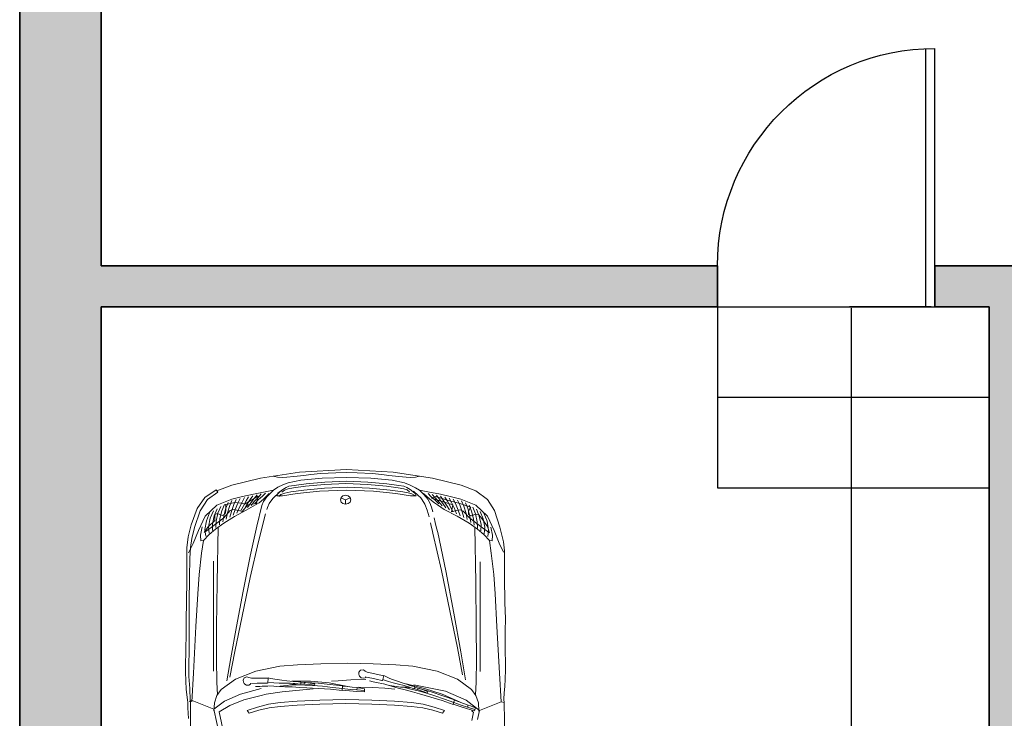
# Model space of a CAD drawing. Units: inches. Extents: x -5 to 482, y -460 to 66.
# Tile 9 of 31: x 33 to 142, y -329 to -252. Entities that reach past the tile are written whole.
import ezdxf

# ---------------------------------------------------------------- set-up
doc = ezdxf.new("R2010")
doc.units = ezdxf.units.IN
doc.header["$MEASUREMENT"] = 0
for name, color, linetype, lineweight in [('A-ANNO-DIMS', 2, 'Continuous', 18), ('A-DOOR', 3, 'Continuous', 25), ('A-EQPM-VEHI', 8, 'Continuous', 13), ('A-FLOR-STRS', 7, 'Continuous', 25), ('A-WALL', 7, 'Continuous', 35), ('A-WALL-PATT', 152, 'Continuous', 13)]:
    doc.layers.add(name, color=color, linetype=linetype, lineweight=lineweight)
doc.styles.get("Standard").update_dxf_attribs({"font": 'arial.ttf'})
doc.dimstyles.get("Standard").update_dxf_attribs({"dimtxt": 0.18, "dimasz": 0.18, "dimexe": 0.18, "dimexo": 0.0625, "dimgap": 0.09, "dimtad": 0, "dimtih": 1, "dimtoh": 1, "dimdec": 0, "dimzin": 0, "dimdsep": 46, "dimlunit": 3, "dimtxsty": 'Standard', "dimcen": 0.09, "dimadec": 0, "dimazin": 0, "dimtfac": 1, "dimtdec": 0, "dimtofl": 0, "dimtmove": 0, "dimatfit": 3, "dimfxl": 1, "dimtolj": 1, "dimtzin": 0, "dimarcsym": 0})

# ---------------------------------------------------------------- blocks, each defined once
blk = doc.blocks.new('*D18')
at = {"layer": 'A-ANNO-DIMS', "color": 0, "lineweight": -2, "transparency": 16777216}
for p, q in [((144.44, -144.35), (144.56, -144.35)), ((144.38, -144.53), (144.38, -208.69)), ((144.38, -279.17), (144.38, -215)), ((144.44, -279.35), (144.56, -279.35))]:
    blk.add_line(p, q, dxfattribs=at)
at = {"layer": 'A-ANNO-DIMS', "color": 0, "transparency": 16777216}
for points in [[(144.35, -144.53), (144.41, -144.53), (144.38, -144.35)], [(144.35, -279.17), (144.41, -279.17), (144.38, -279.35)]]:
    blk.add_solid(points, dxfattribs=at)
at = {"layer": 'Defpoints', "color": 0, "transparency": 16777216}
for p in [(144.38, -144.35), (144.38, -144.35), (144.38, -279.35)]:
    blk.add_point(p, dxfattribs=at)
at = {"layer": 'A-ANNO-DIMS', "color": 0, "transparency": 16777216, "insert": (144.38, -211.85), "char_height": 6, "attachment_point": 5}
blk.add_mtext('\\A1;11\'-3"', dxfattribs=at)
blk = doc.blocks.new('*D21')
at = {"layer": 'A-ANNO-DIMS', "color": 0, "lineweight": -2, "transparency": 16777216}
for p, q in [((133.45, -283.85), (124.45, -283.85)), ((124.63, -284.03), (124.63, -345.73)), ((124.63, -413.74), (124.63, -352.04)), ((124.69, -413.92), (124.81, -413.92))]:
    blk.add_line(p, q, dxfattribs=at)
at = {"layer": 'A-ANNO-DIMS', "color": 0, "transparency": 16777216}
for points in [[(124.6, -284.03), (124.66, -284.03), (124.63, -283.85)], [(124.6, -413.74), (124.66, -413.74), (124.63, -413.92)]]:
    blk.add_solid(points, dxfattribs=at)
at = {"layer": 'Defpoints', "color": 0, "transparency": 16777216}
for p in [(124.63, -283.85), (133.51, -283.85), (124.63, -413.92)]:
    blk.add_point(p, dxfattribs=at)
at = {"layer": 'A-ANNO-DIMS', "color": 0, "transparency": 16777216, "insert": (124.63, -348.88), "char_height": 6, "attachment_point": 5}
blk.add_mtext('\\A1;10\'-10"', dxfattribs=at)
blk = doc.blocks.new('DOOR-SWING-24IN')
for p, q in [((24, 1), (0, 1)), ((24, 0), (0, 0))]:
    blk.add_line(p, q)
blk.add_arc((24, 0), 24, 90, 180)

msp = doc.modelspace()

# ---------------------------------------------------------------- hatches: boundary and pattern name
at = {"layer": 'A-WALL-PATT'}
h = msp.add_hatch(color=256, dxfattribs=at)
h.dxf.hatch_style = 1
h.paths.add_polyline_path([(149.38, -412.85), (144.38, -412.85), (144.38, -283.85), (144.38, -279.35), (133.88, -279.35), (133.88, -283.85), (139.88, -283.85), (139.88, -412.85), (133.51, -412.85), (133.51, -413.92), (102.65, -413.92), (102.65, -421.02), (133.51, -421.02), (133.51, -421.85), (149.38, -421.85)])
h.paths.add_polyline_path([(226.05, -412.85), (218.88, -412.85), (218.88, -350.85), (262.88, -350.85), (262.88, -386.85), (267.38, -386.85), (267.38, -283.85), (270.38, -283.85), (270.38, -279.35), (244.88, -279.35), (244.88, -283.85), (262.88, -283.85), (262.88, -346.35), (218.88, -346.35), (218.88, -283.85), (220.88, -283.85), (220.88, -279.35), (214.38, -279.35), (214.38, -283.85), (214.38, -412.85), (209.38, -412.85), (209.38, -421.85), (226.05, -421.85)])
h.paths.add_polyline_path([(315.81, -412.85), (250.05, -412.85), (250.05, -421.85), (315.81, -421.85)])
h.paths.add_polyline_path([(430.38, -378.35), (421.38, -378.35), (421.38, -412.85), (375.81, -412.85), (375.81, -421.85), (430.38, -421.85)])
h.paths.add_polyline_path([(78.69, -413.92), (47.68, -413.92), (47.68, -412.85), (41.88, -412.85), (41.88, -283.85), (109.88, -283.85), (109.88, -279.35), (41.88, -279.35), (41.88, -241.85), (32.88, -241.85), (32.88, -421.85), (47.68, -421.85), (47.68, -421.02), (78.69, -421.02)])
h.paths.add_polyline_path([(41.88, -144.35), (154.38, -144.35), (154.38, -137.85), (149.88, -137.85), (149.88, -139.85), (41.88, -139.85), (41.88, -97.85), (32.88, -97.85), (32.88, -181.85), (41.88, -181.85)])
h.paths.add_polyline_path([(430.38, -241.85), (421.38, -241.85), (421.38, -279.35), (309.38, -279.35), (309.38, -170.35), (304.88, -170.35), (304.88, -279.35), (294.38, -279.35), (294.38, -283.85), (421.38, -283.85), (421.38, -318.35), (430.38, -318.35)])
h.paths.add_polyline_path([(430.38, -119.85), (421.38, -119.85), (421.38, -139.85), (419.38, -139.85), (419.38, -144.35), (421.38, -144.35), (421.38, -181.85), (430.38, -181.85)])
h.paths.add_polyline_path([(395.38, -139.85), (377.38, -139.85), (377.38, -75.85), (421.38, -75.85), (421.38, -95.85), (430.38, -95.85), (430.38, -45.6), (421.38, -45.6), (421.38, -71.35), (377.38, -71.35), (377.38, -22.85), (372.88, -22.85), (372.88, -139.85), (242.88, -139.85), (242.88, -137.85), (238.38, -137.85), (238.38, -144.35), (304.88, -144.35), (304.88, -146.35), (309.38, -146.35), (309.38, -144.35), (395.38, -144.35)])
h.paths.add_polyline_path([(65.88, 13.15), (32.88, 13.15), (32.88, -37.85), (41.88, -37.85), (41.88, 4.15), (65.88, 4.15)])
h.paths.add_polyline_path([(166.38, 13.15), (125.88, 13.15), (125.88, 4.15), (149.88, 4.15), (149.88, -113.85), (154.38, -113.85), (154.38, 4.15), (166.38, 4.15)])
h.paths.add_polyline_path([(277.88, 13.15), (226.38, 13.15), (226.38, 4.15), (238.38, 4.15), (238.38, -113.85), (242.88, -113.85), (242.88, 4.15), (277.88, 4.15)])
h.paths.add_polyline_path([(430.38, 13.15), (337.88, 13.15), (337.88, 4.15), (372.88, 4.15), (372.88, 1.15), (377.38, 1.15), (377.38, 4.15), (421.38, 4.15), (421.38, -21.6), (430.38, -21.6)])

# ---------------------------------------------------------------- linework, layer by layer
at = {"layer": 'A-DOOR'}
msp.add_line((132.88, -283.85), (132.88, -279.35), dxfattribs=at)
at = {"layer": 'A-EQPM-VEHI'}
for p, q in [((68.93, -301.81), (63.77, -302.12)), ((68.93, -301.81), (74.1, -302.12)), ((59.45, -302.78), (56.29, -303.55)), ((63.77, -302.12), (59.45, -302.78)), ((60.86, -302.56), (61.32, -302.65)), ((61.32, -302.65), (61.86, -302.68)), ((61.86, -302.68), (62.35, -302.66)), ((62.35, -302.66), (63.14, -302.58)), ((62.52, -303.27), (63.89, -303)), ((63.14, -302.58), (64.25, -302.46)), ((63.89, -303), (66.26, -302.78)), ((64.25, -302.46), (65.02, -302.36)), ((65.02, -302.36), (66.08, -302.27)), ((66.08, -302.27), (67.76, -302.19)), ((66.26, -302.78), (68.93, -302.69)), ((66.56, -303.2), (68.93, -303.1)), ((67.76, -302.19), (68.93, -302.15)), ((70.11, -302.19), (68.93, -302.15)), ((68.93, -302.69), (71.61, -302.78)), ((68.93, -303.1), (71.31, -303.2)), ((71.79, -302.27), (70.11, -302.19)), ((71.61, -302.78), (73.98, -303)), ((72.85, -302.36), (71.79, -302.27)), ((73.62, -302.46), (72.85, -302.36)), ((74.73, -302.58), (73.62, -302.46)), ((73.98, -303), (75.35, -303.27)), ((74.1, -302.12), (78.42, -302.78)), ((75.52, -302.66), (74.73, -302.58)), ((76.01, -302.68), (75.52, -302.66)), ((76.55, -302.65), (76.01, -302.68)), ((77.01, -302.56), (76.55, -302.65)), ((78.42, -302.78), (81.58, -303.55)), ((53.32, -304.91), (54.57, -304.06)), ((54.57, -304.06), (54.74, -304.3)), ((56.29, -303.55), (54.64, -304.18)), ((60.89, -304.11), (60.14, -304.83)), ((60.16, -304.25), (60.89, -304.11)), ((60.89, -304.11), (61.36, -303.77)), ((61.36, -303.77), (61.9, -303.51)), ((61.37, -304.42), (61.91, -304.01)), ((61.82, -304.33), (62.1, -304.09)), ((61.9, -303.51), (62.52, -303.27)), ((61.91, -304.01), (62.27, -303.79)), ((62.1, -304.09), (62.49, -303.94)), ((62.27, -303.79), (62.59, -303.66)), ((62.49, -303.94), (63.11, -303.83)), ((62.59, -303.66), (63.16, -303.57)), ((62.81, -304.29), (64.24, -304.11)), ((63.11, -303.83), (64.42, -303.66)), ((63.16, -303.57), (64.48, -303.4)), ((65.96, -304.22), (63.51, -304.47)), ((64.24, -304.11), (66.53, -303.87)), ((64.42, -303.66), (66.51, -303.46)), ((64.48, -303.4), (66.56, -303.2)), ((68.9, -304.11), (65.96, -304.22)), ((66.51, -303.46), (68.88, -303.36)), ((66.53, -303.87), (69.01, -303.75)), ((68.88, -303.36), (71.26, -303.46)), ((71.91, -304.22), (68.9, -304.11)), ((69.01, -303.75), (71.49, -303.87)), ((71.26, -303.46), (73.34, -303.66)), ((71.31, -303.2), (73.39, -303.4)), ((71.49, -303.87), (73.75, -304.11)), ((74.37, -304.47), (71.91, -304.22)), ((73.34, -303.66), (74.66, -303.83)), ((73.39, -303.4), (74.71, -303.57)), ((73.75, -304.11), (75.17, -304.29)), ((74.66, -303.83), (75.26, -303.93)), ((74.71, -303.57), (75.28, -303.66)), ((75.26, -303.93), (75.62, -304.06)), ((75.28, -303.66), (75.6, -303.79)), ((75.35, -303.27), (75.98, -303.54)), ((75.6, -303.79), (75.96, -304.01)), ((75.62, -304.06), (75.89, -304.26)), ((75.96, -304.01), (76.5, -304.42)), ((75.98, -303.54), (76.54, -303.82)), ((76.35, -304.2), (76.82, -304.63)), ((76.54, -303.82), (76.98, -304.11)), ((76.98, -304.11), (77.44, -304.55)), ((76.98, -304.11), (77.9, -304.28)), ((81.58, -303.55), (83.23, -304.18)), ((83.23, -304.18), (84.49, -305.12)), ((52.46, -306.1), (53.32, -304.91)), ((53.59, -305.14), (52.79, -306.38)), ((54.74, -304.3), (53.59, -305.14)), ((54.65, -305.76), (56.3, -305.09)), ((56.28, -305.23), (56.05, -305.79)), ((56.3, -305.09), (57.48, -304.79)), ((56.75, -305.12), (56.5, -305.66)), ((57.21, -305.02), (56.95, -305.53)), ((57.68, -304.92), (57.41, -305.4)), ((57.48, -304.79), (58.67, -304.54)), ((57.86, -305.27), (57.52, -305.88)), ((57.68, -305.63), (59.19, -304.75)), ((58.14, -304.82), (57.86, -305.27)), ((58.31, -305.14), (57.95, -305.69)), ((58.6, -304.71), (58.31, -305.14)), ((58.77, -305.01), (58.37, -305.51)), ((58.8, -305.32), (58.43, -305.78)), ((58.67, -304.54), (60.16, -304.25)), ((59.07, -304.61), (58.77, -305.01)), ((59.22, -304.88), (58.8, -305.32)), ((59.23, -305.14), (58.82, -305.57)), ((59.19, -304.75), (59, -305.55)), ((59.53, -304.51), (59.22, -304.88)), ((59.67, -304.75), (59.23, -305.14)), ((59.31, -305.48), (59.79, -305.1)), ((60, -304.41), (59.67, -304.75)), ((60.14, -304.83), (59.77, -305.35)), ((59.79, -305.1), (60.42, -304.48)), ((60.82, -305), (60.4, -305.57)), ((61.6, -304.29), (60.82, -305)), ((61.24, -304.72), (61.37, -304.42)), ((61.87, -304.72), (61.24, -304.72)), ((61.46, -304.8), (61.69, -304.58)), ((61.69, -304.58), (62.14, -304.42)), ((63.51, -304.47), (61.87, -304.72)), ((62.14, -304.42), (62.81, -304.29)), ((68.27, -305.15), (68.34, -304.9)), ((68.34, -305.4), (68.27, -305.15)), ((68.84, -305.15), (68.32, -304.93)), ((68.34, -304.9), (68.55, -304.72)), ((68.55, -304.72), (68.84, -304.65)), ((68.84, -304.65), (69.12, -304.72)), ((69.35, -304.93), (68.84, -305.15)), ((68.84, -305.15), (68.84, -305.65)), ((69.12, -304.72), (69.33, -304.9)), ((69.33, -304.9), (69.41, -305.15)), ((69.41, -305.15), (69.33, -305.4)), ((76, -304.72), (74.37, -304.47)), ((75.17, -304.29), (75.74, -304.39)), ((75.74, -304.39), (76.15, -304.5)), ((76.62, -304.72), (76, -304.72)), ((76.15, -304.5), (76.49, -304.68)), ((76.5, -304.42), (76.62, -304.72)), ((76.82, -304.63), (77.14, -304.94)), ((77.14, -304.94), (77.31, -305.17)), ((77.31, -305.17), (77.57, -305.65)), ((77.44, -304.55), (77.75, -304.86)), ((78.13, -305.1), (77.45, -304.48)), ((77.75, -304.86), (77.92, -305.09)), ((77.9, -304.28), (79.3, -304.55)), ((77.92, -305.09), (78.14, -305.5)), ((77.94, -304.46), (78.26, -304.8)), ((78.65, -305.48), (78.13, -305.1)), ((78.26, -304.8), (78.71, -305.19)), ((78.75, -304.8), (78.34, -304.98)), ((78.34, -304.98), (80.67, -305.7)), ((78.4, -304.56), (78.72, -304.93)), ((78.71, -305.19), (79.12, -305.62)), ((78.72, -304.93), (79.14, -305.38)), ((80.47, -305.3), (78.75, -304.8)), ((78.87, -304.66), (79.17, -305.06)), ((79.17, -305.06), (79.56, -305.56)), ((79.3, -304.55), (80.39, -304.79)), ((79.33, -304.77), (79.62, -305.19)), ((79.62, -305.19), (79.99, -305.74)), ((79.8, -304.87), (80.08, -305.32)), ((80.08, -305.32), (80.42, -305.93)), ((80.26, -304.97), (80.53, -305.45)), ((80.39, -304.79), (81.57, -305.09)), ((80.78, -305.38), (80.47, -305.3)), ((80.73, -305.07), (80.98, -305.58)), ((81.19, -305.18), (81.44, -305.72)), ((81.57, -305.09), (83.22, -305.76)), ((81.65, -305.28), (81.89, -305.85)), ((84.49, -305.12), (85.26, -306.35)), ((51.81, -307.91), (52.46, -306.1)), ((52.79, -306.38), (52.16, -308.21)), ((53.36, -306.98), (54.65, -305.76)), ((54.25, -306.37), (53.9, -307.2)), ((54.66, -306.14), (54.33, -306.92)), ((55.06, -305.91), (54.76, -306.64)), ((55.19, -306.36), (54.98, -307.22)), ((55.47, -305.69), (55.19, -306.36)), ((55.62, -306.08), (55.39, -306.92)), ((56.1, -306.35), (55.4, -307.14)), ((55.54, -306.72), (55.61, -306.32)), ((55.6, -305.68), (56.67, -305.46)), ((55.61, -305.89), (55.6, -305.68)), ((55.61, -306.32), (55.61, -305.89)), ((55.88, -305.46), (55.62, -306.08)), ((56.05, -305.79), (55.81, -306.61)), ((56.4, -306.21), (56.1, -306.35)), ((56.5, -305.66), (56.24, -306.43)), ((57.05, -306.34), (56.4, -306.21)), ((56.66, -306.24), (56.45, -306.85)), ((56.6, -307.01), (57.87, -306.3)), ((56.95, -305.53), (56.66, -306.24)), ((56.67, -305.46), (57.41, -305.54)), ((57.09, -306.06), (56.85, -306.64)), ((57.42, -306.44), (57.05, -306.34)), ((57.41, -305.4), (57.09, -306.06)), ((57.52, -305.88), (57.24, -306.42)), ((57.41, -305.54), (57.68, -305.63)), ((58.04, -305.73), (57.42, -306.44)), ((57.95, -305.69), (57.64, -306.21)), ((57.87, -306.3), (58.9, -305.73)), ((58.37, -305.51), (58.03, -306)), ((59, -305.55), (58.04, -305.73)), ((58.9, -305.73), (59.31, -305.48)), ((59.6, -305.78), (59.03, -308.05)), ((59.77, -305.35), (59.6, -305.78)), ((60.21, -306.01), (60.14, -306.22)), ((60.4, -305.57), (60.21, -306.01)), ((68.55, -305.58), (68.34, -305.4)), ((68.84, -305.65), (68.55, -305.58)), ((69.12, -305.58), (68.84, -305.65)), ((69.33, -305.4), (69.12, -305.58)), ((77.57, -305.65), (77.84, -306.3)), ((77.84, -306.3), (78.05, -307.03)), ((78.14, -305.5), (78.32, -305.96)), ((78.32, -305.96), (78.48, -306.47)), ((78.97, -305.73), (78.65, -305.48)), ((79.73, -306.21), (78.97, -305.73)), ((79.14, -305.38), (79.51, -305.83)), ((79.56, -305.56), (79.9, -306.05)), ((81.14, -306.96), (79.73, -306.21)), ((79.99, -305.74), (80.3, -306.26)), ((80.42, -305.93), (80.69, -306.48)), ((80.67, -305.7), (80.52, -306.5)), ((80.52, -306.5), (80.88, -306.39)), ((80.53, -305.45), (80.85, -306.11)), ((81.57, -305.6), (80.78, -305.38)), ((80.85, -306.11), (81.09, -306.69)), ((80.88, -306.39), (81.54, -306.27)), ((80.98, -305.58), (81.27, -306.29)), ((81.27, -306.29), (81.48, -306.91)), ((81.44, -305.72), (81.7, -306.48)), ((81.54, -306.27), (81.83, -306.4)), ((82.67, -305.98), (81.57, -305.6)), ((81.83, -306.4), (82.54, -307.19)), ((81.89, -305.85), (82.13, -306.66)), ((82.06, -305.51), (82.32, -306.13)), ((82.32, -306.13), (82.54, -306.97)), ((82.41, -306.44), (82.57, -306.12)), ((82.47, -305.74), (82.75, -306.41)), ((82.57, -306.12), (82.67, -305.98)), ((82.75, -306.41), (82.96, -307.27)), ((82.87, -305.97), (83.18, -306.69)), ((83.22, -305.76), (84.51, -306.98)), ((83.28, -306.2), (83.6, -306.97)), ((85.26, -306.35), (85.86, -308.17)), ((52.61, -308.55), (53.36, -306.98)), ((53.48, -307.48), (53.32, -308.44)), ((53.84, -306.6), (53.48, -307.48)), ((53.63, -308.16), (54.42, -307.43)), ((53.9, -307.2), (53.73, -308.14)), ((55.4, -307.14), (53.99, -308.21)), ((54.33, -306.92), (54.15, -307.83)), ((54.4, -306.77), (54.72, -306.68)), ((54.42, -307.43), (54.4, -306.77)), ((54.76, -306.64), (54.56, -307.53)), ((54.72, -306.68), (55.22, -306.88)), ((54.98, -307.22), (54.91, -307.91)), ((55.22, -306.88), (55.54, -306.72)), ((55.39, -306.92), (55.29, -307.6)), ((55.39, -307.73), (56.6, -307.01)), ((55.81, -306.61), (55.67, -307.28)), ((56.24, -306.43), (56.06, -307.07)), ((59.99, -306.7), (59.22, -309.74)), ((78.63, -307.16), (78.74, -307.66)), ((82.48, -307.73), (81.14, -306.96)), ((81.7, -306.48), (81.88, -307.12)), ((82.13, -306.66), (82.27, -307.34)), ((82.4, -306.77), (82.41, -306.44)), ((82.71, -306.93), (82.4, -306.77)), ((82.54, -306.97), (82.65, -307.65)), ((82.54, -307.19), (83.95, -308.26)), ((83.22, -306.74), (82.71, -306.93)), ((82.96, -307.27), (83.02, -307.96)), ((83.18, -306.69), (83.37, -307.58)), ((83.54, -306.82), (83.22, -306.74)), ((83.89, -307.23), (83.54, -306.82)), ((83.6, -306.97), (83.79, -307.88)), ((83.69, -306.43), (84.03, -307.25)), ((84.5, -308.09), (83.89, -307.23)), ((84.03, -307.25), (84.21, -308.19)), ((84.09, -306.65), (84.46, -307.53)), ((84.51, -306.98), (85.24, -308.54)), ((51.48, -309.25), (51.81, -307.91)), ((52.16, -308.21), (51.87, -309.42)), ((52.01, -309.98), (52.61, -308.55)), ((53.01, -308.14), (52.82, -309.05)), ((53.22, -308.75), (53.63, -308.16)), ((53.99, -308.21), (53.22, -308.75)), ((53.32, -308.44), (53.41, -309.16)), ((53.73, -308.14), (53.78, -308.85)), ((53.78, -309), (54.47, -308.38)), ((54.15, -307.83), (54.16, -308.53)), ((54.47, -308.38), (55.39, -307.73)), ((54.56, -307.53), (54.54, -308.22)), ((54.78, -308.17), (54.66, -314.28)), ((59.03, -308.05), (58.31, -311.37)), ((78.21, -307.71), (78.29, -308.08)), ((78.29, -308.08), (78.38, -308.46)), ((78.38, -308.46), (78.47, -308.83)), ((78.74, -307.66), (78.89, -308.27)), ((78.89, -308.27), (79.01, -308.77)), ((83.4, -308.38), (82.48, -307.73)), ((83.09, -308.17), (83.2, -314.28)), ((83.37, -307.58), (83.4, -308.27)), ((84.09, -309), (83.4, -308.38)), ((83.79, -307.88), (83.78, -308.59)), ((83.95, -308.26), (84.72, -308.8)), ((84.21, -308.19), (84.15, -308.9)), ((84.46, -307.53), (84.62, -308.49)), ((84.72, -308.8), (84.5, -308.09)), ((84.62, -308.49), (84.53, -309.21)), ((84.87, -308.17), (85.05, -309.07)), ((85.24, -308.54), (85.8, -309.93)), ((85.86, -308.17), (86.27, -309.81)), ((51.33, -310.47), (51.48, -309.25)), ((51.87, -309.42), (51.74, -310.43)), ((52.82, -309.05), (52.85, -309.68)), ((52.85, -309.68), (53.16, -309.65)), ((53.16, -309.65), (52.95, -311.05)), ((53.16, -309.65), (53.78, -309)), ((78.47, -308.83), (79.41, -312.97)), ((79.01, -308.77), (79.89, -313.01)), ((84.71, -309.65), (84.09, -309)), ((84.71, -309.65), (84.92, -311.05)), ((85.01, -309.69), (84.71, -309.65)), ((85.05, -309.07), (85.01, -309.69)), ((51.31, -311.81), (51.33, -310.47)), ((51.5, -311), (52.01, -309.98)), ((51.74, -310.43), (51.66, -311.64)), ((59.22, -309.74), (58.31, -313.72)), ((85.8, -309.93), (86.28, -310.95)), ((86.27, -309.81), (86.39, -310.77)), ((51.31, -313.83), (51.31, -311.81)), ((51.66, -311.64), (51.61, -313.7)), ((52.95, -311.05), (52.68, -313.41)), ((58.31, -311.37), (57.54, -315.23)), ((84.92, -311.05), (85.19, -313.41)), ((86.39, -310.77), (86.37, -311.65)), ((86.37, -311.65), (86.38, -313.71)), ((54.25, -324.05), (54.25, -311.91)), ((83.71, -324.09), (83.71, -311.99)), ((51.27, -316.59), (51.31, -313.83)), ((51.61, -313.7), (51.58, -316.54)), ((52.68, -313.41), (52.52, -315.53)), ((58.31, -313.72), (57.41, -317.99)), ((79.41, -312.97), (80.36, -317.42)), ((79.89, -313.01), (80.78, -317.67)), ((85.19, -313.41), (85.35, -315.53)), ((86.38, -313.71), (86.43, -316.54)), ((54.66, -314.28), (54.6, -319.13)), ((83.2, -314.28), (83.26, -319.13)), ((52.52, -315.53), (52.33, -319.12)), ((57.54, -315.23), (56.8, -319.15)), ((85.35, -315.53), (85.54, -319.12)), ((51.24, -318.27), (51.27, -316.59)), ((51.58, -316.54), (51.57, -318.27)), ((86.43, -316.54), (86.47, -318.27)), ((51.24, -319.71), (51.24, -318.27)), ((51.57, -318.27), (51.57, -319.7)), ((57.41, -317.99), (56.61, -321.89)), ((80.36, -317.42), (81.18, -321.49)), ((80.78, -317.67), (81.55, -321.95)), ((86.47, -318.27), (86.46, -319.66)), ((52.33, -319.12), (52.04, -324.3)), ((54.6, -319.13), (54.59, -322.77)), ((56.8, -319.15), (56.17, -322.61)), ((83.26, -319.13), (83.27, -322.77)), ((85.54, -319.12), (85.83, -324.3)), ((51.22, -321.92), (51.24, -319.71)), ((51.57, -319.7), (51.57, -321.9)), ((86.46, -319.66), (86.45, -321.79)), ((81.18, -321.49), (81.75, -324.48)), ((51.19, -323.33), (51.22, -321.92)), ((51.57, -321.9), (51.55, -323.31)), ((56.17, -322.61), (55.74, -325.14)), ((56.61, -321.89), (56.05, -324.74)), ((81.55, -321.95), (82.07, -325.04)), ((86.45, -321.79), (86.47, -323.17)), ((51.18, -324.13), (51.19, -323.33)), ((51.55, -323.31), (51.55, -324.65)), ((54.59, -322.77), (54.63, -325.27)), ((61.59, -323.5), (58.93, -324.06)), ((63.52, -323.35), (61.59, -323.5)), ((66.11, -323.26), (63.52, -323.35)), ((69.03, -323.18), (66.11, -323.26)), ((71.9, -323.26), (69.03, -323.18)), ((74.39, -323.35), (71.9, -323.26)), ((76.28, -323.5), (74.39, -323.35)), ((78.94, -324.06), (76.28, -323.5)), ((83.27, -322.77), (83.24, -325.27)), ((86.47, -323.17), (86.48, -323.93)), ((51.2, -325.18), (51.18, -324.13)), ((51.55, -324.65), (51.65, -325.96)), ((52.04, -324.3), (51.87, -327.46)), ((58.93, -324.06), (56.68, -324.96)), ((57.52, -325.07), (57.64, -324.81)), ((57.64, -324.81), (57.96, -324.69)), ((57.96, -324.69), (58.18, -324.78)), ((58.18, -324.78), (58.44, -324.85)), ((58.44, -324.85), (60.3, -324.84)), ((60.31, -324.81), (60.27, -325.4)), ((60.55, -324.86), (60.31, -324.81)), ((60.8, -324.92), (60.55, -324.86)), ((70.29, -324.39), (70.3, -324.18)), ((70.33, -324.53), (70.29, -324.39)), ((70.3, -324.18), (70.47, -323.95)), ((70.39, -324.63), (70.33, -324.53)), ((70.55, -324.79), (70.39, -324.63)), ((70.47, -323.95), (70.81, -323.91)), ((70.82, -324.85), (70.55, -324.79)), ((70.81, -323.91), (71, -324.05)), ((71, -324.79), (70.82, -324.85)), ((71, -324.05), (71.24, -324.17)), ((71.03, -324.73), (71, -324.79)), ((71.06, -324.7), (71.03, -324.73)), ((71.75, -324.85), (71.11, -324.72)), ((71.24, -324.17), (73.06, -324.58)), ((72.22, -324.95), (71.75, -324.85)), ((73.07, -324.55), (72.9, -325.12)), ((73.36, -324.68), (73.07, -324.55)), ((73.71, -324.86), (73.36, -324.68)), ((74, -324.98), (73.71, -324.86)), ((81.19, -324.96), (78.94, -324.06)), ((85.83, -324.3), (86, -327.46)), ((86.48, -323.93), (86.46, -324.94)), ((51.26, -326.04), (51.2, -325.18)), ((51.65, -325.96), (51.7, -327.3)), ((54.63, -325.27), (54.71, -326.68)), ((56.68, -324.96), (55.12, -326.07)), ((59.53, -325.96), (57.23, -326.59)), ((57.56, -325.28), (57.52, -325.07)), ((57.64, -325.41), (57.56, -325.28)), ((57.71, -325.49), (57.64, -325.41)), ((57.9, -325.61), (57.71, -325.49)), ((58.18, -325.6), (57.9, -325.61)), ((58.34, -325.5), (58.18, -325.6)), ((58.36, -325.44), (58.34, -325.5)), ((58.38, -325.41), (58.36, -325.44)), ((59.08, -325.4), (58.44, -325.41)), ((58.9, -325.75), (59.14, -325.75)), ((59.57, -325.39), (59.08, -325.4)), ((59.14, -325.75), (59.39, -325.74)), ((59.39, -325.74), (59.63, -325.73)), ((60.21, -325.38), (59.57, -325.39)), ((59.63, -325.73), (59.84, -325.72)), ((59.84, -325.72), (60.06, -325.72)), ((60.06, -325.72), (60.27, -325.71)), ((60.35, -325.7), (62.15, -325.8)), ((60.94, -325.34), (60.36, -325.3)), ((61.04, -324.96), (60.8, -324.92)), ((61.5, -325.38), (60.94, -325.34)), ((61.79, -325.06), (61.04, -324.96)), ((61.21, -325.74), (62.38, -325.63)), ((62.08, -325.38), (61.5, -325.38)), ((62.36, -325.14), (61.79, -325.06)), ((62.72, -325.38), (62.08, -325.38)), ((62.15, -325.8), (62.96, -325.81)), ((63.06, -325.2), (62.36, -325.14)), ((62.71, -325.57), (62.38, -325.63)), ((63.52, -325.59), (62.69, -325.57)), ((63.04, -325.5), (62.71, -325.57)), ((63.24, -325.42), (62.72, -325.38)), ((64.97, -325.18), (62.9, -325.16)), ((62.96, -325.81), (63.77, -325.85)), ((63.37, -325.48), (63.04, -325.5)), ((63.34, -325.22), (63.06, -325.2)), ((63.89, -325.5), (63.24, -325.42)), ((63.63, -325.25), (63.34, -325.22)), ((64.36, -325.6), (63.52, -325.59)), ((63.91, -325.27), (63.63, -325.25)), ((63.77, -325.85), (64.57, -325.9)), ((63.88, -325.46), (64.4, -325.49)), ((63.91, -325.29), (63.89, -325.5)), ((64.41, -325.31), (63.9, -325.28)), ((64.3, -325.3), (64.28, -325.48)), ((65.19, -325.63), (64.36, -325.6)), ((64.4, -325.49), (64.91, -325.55)), ((64.93, -325.38), (64.41, -325.31)), ((64.45, -325.33), (65.8, -325.39)), ((64.57, -325.9), (65.87, -325.96)), ((64.91, -325.55), (65.42, -325.62)), ((65.44, -325.45), (64.93, -325.38)), ((67.04, -325.36), (64.97, -325.18)), ((66.29, -325.73), (65.19, -325.63)), ((65.44, -325.45), (65.41, -325.62)), ((65.8, -325.39), (67.15, -325.53)), ((65.87, -325.96), (67.18, -326.05)), ((67.39, -325.85), (66.29, -325.73)), ((69.08, -325.77), (67.04, -325.36)), ((67.15, -325.53), (68.5, -325.68)), ((68.03, -325.12), (67.28, -325.16)), ((68.49, -325.96), (67.39, -325.85)), ((69.43, -325.04), (68.03, -325.12)), ((68.5, -325.68), (68.48, -326.16)), ((69.37, -326.08), (68.48, -325.97)), ((68.5, -325.72), (69.04, -325.77)), ((69.04, -325.77), (69.57, -325.82)), ((71.06, -324.99), (69.43, -325.04)), ((69.57, -325.82), (70.11, -325.88)), ((70.11, -325.89), (70.09, -326.13)), ((70.11, -325.89), (70.39, -325.92)), ((71.82, -325.85), (70.3, -325.82)), ((70.39, -325.92), (70.66, -325.96)), ((70.66, -325.96), (70.94, -326)), ((71.49, -325.15), (71.89, -325.24)), ((73.16, -325.93), (71.82, -325.85)), ((71.89, -325.24), (72.44, -325.35)), ((72.85, -325.08), (72.22, -324.95)), ((72.44, -325.35), (72.83, -325.42)), ((72.92, -325.43), (74.65, -325.93)), ((73.57, -325.21), (73.01, -325.04)), ((74.29, -326.04), (73.16, -325.93)), ((74.1, -325.37), (73.57, -325.21)), ((73.74, -325.66), (74.91, -325.82)), ((74.58, -325.17), (74, -324.98)), ((74.67, -325.51), (74.1, -325.37)), ((75.08, -325.36), (74.58, -325.17)), ((74.65, -325.93), (75.43, -326.12)), ((75.3, -325.65), (74.67, -325.51)), ((75.24, -325.83), (74.91, -325.82)), ((75.67, -325.55), (75.08, -325.36)), ((76.03, -326.04), (75.22, -325.83)), ((75.57, -325.84), (75.24, -325.83)), ((75.79, -325.81), (75.3, -325.65)), ((77.54, -325.96), (75.51, -325.47)), ((75.9, -325.89), (75.57, -325.84)), ((75.94, -325.63), (75.67, -325.55)), ((76.41, -326.03), (75.79, -325.81)), ((76.21, -325.72), (75.94, -325.63)), ((76.47, -325.81), (76.21, -325.72)), ((79.86, -326.26), (76.39, -325.58)), ((76.47, -325.83), (76.41, -326.03)), ((76.96, -325.96), (76.47, -325.82)), ((76.85, -325.93), (76.79, -326.1)), ((77.45, -326.14), (76.96, -325.96)), ((79.51, -326.6), (77.54, -325.96)), ((82.75, -326.07), (81.19, -324.96)), ((83.24, -325.27), (83.16, -326.68)), ((86.4, -325.77), (86.35, -326.47)), ((86.46, -324.94), (86.4, -325.77)), ((51.33, -326.68), (51.26, -326.04)), ((51.39, -327.23), (51.33, -326.68)), ((54.65, -326.74), (54.37, -327.56)), ((55.12, -326.07), (54.65, -326.74)), ((57.23, -326.59), (55.48, -327.37)), ((59.53, -326.74), (57.61, -327.24)), ((60.06, -326.61), (59.53, -326.74)), ((61.86, -326.33), (60.06, -326.61)), ((65.27, -326.02), (61.86, -326.33)), ((67.18, -326.05), (68.48, -326.19)), ((68.48, -326.16), (69.29, -326.24)), ((69.29, -326.24), (70.1, -326.31)), ((69.37, -326.08), (70.09, -326.13)), ((70.09, -326.13), (70.93, -326.2)), ((70.1, -326.31), (70.92, -326.35)), ((70.94, -326), (70.92, -326.35)), ((75.43, -326.12), (76.21, -326.34)), ((76.84, -326.23), (76.03, -326.04)), ((76.21, -326.34), (76.98, -326.57)), ((76.41, -325.99), (76.9, -326.14)), ((77.65, -326.45), (76.84, -326.23)), ((76.9, -326.14), (77.39, -326.31)), ((76.98, -326.57), (78.23, -326.92)), ((76.99, -325.99), (78.29, -326.35)), ((77.39, -326.31), (77.87, -326.49)), ((77.93, -326.33), (77.45, -326.14)), ((78.7, -326.79), (77.65, -326.45)), ((77.93, -326.33), (77.86, -326.49)), ((78.23, -326.92), (79.49, -327.31)), ((78.29, -326.35), (79.58, -326.8)), ((79.74, -327.15), (78.7, -326.79)), ((81.4, -327.46), (79.51, -326.6)), ((79.58, -326.8), (80.86, -327.24)), ((82.16, -327.26), (79.86, -326.26)), ((83.22, -326.74), (82.75, -326.07)), ((83.5, -327.56), (83.22, -326.74)), ((86.35, -326.47), (86.32, -327.17)), ((51.42, -327.53), (51.39, -327.23)), ((51.45, -328.11), (51.42, -327.53)), ((51.5, -329.28), (51.45, -328.11)), ((51.57, -327.4), (51.91, -327.29)), ((51.7, -327.3), (51.72, -327.33)), ((51.72, -327.69), (51.71, -328.75)), ((51.72, -327.33), (51.72, -327.36)), ((51.72, -327.36), (51.73, -327.39)), ((51.73, -327.39), (51.72, -327.69)), ((51.91, -327.29), (54.29, -328.27)), ((55.48, -327.37), (54.29, -328.27)), ((54.37, -327.56), (54.31, -328.47)), ((56.06, -327.85), (54.88, -328.54)), ((57.61, -327.24), (56.06, -327.85)), ((59.11, -328.02), (57.97, -328.4)), ((60.33, -327.72), (59.11, -328.02)), ((59.28, -328.36), (60.39, -328.12)), ((61.62, -327.51), (60.33, -327.72)), ((60.39, -328.12), (61.62, -327.95)), ((63.5, -327.36), (61.62, -327.51)), ((61.62, -327.95), (63.5, -327.8)), ((66, -327.26), (63.5, -327.36)), ((63.5, -327.8), (66, -327.7)), ((68.87, -327.19), (66, -327.26)), ((66, -327.7), (68.87, -327.63)), ((71.74, -327.26), (68.87, -327.19)), ((68.87, -327.63), (71.74, -327.7)), ((74.24, -327.36), (71.74, -327.26)), ((71.74, -327.7), (74.24, -327.8)), ((76.13, -327.51), (74.24, -327.36)), ((74.24, -327.8), (76.13, -327.95)), ((77.41, -327.72), (76.13, -327.51)), ((76.13, -327.95), (77.35, -328.12)), ((77.35, -328.12), (78.46, -328.36)), ((78.63, -328.02), (77.41, -327.72)), ((79.77, -328.4), (78.63, -328.02)), ((79.49, -327.31), (80.72, -327.74)), ((80.78, -327.51), (79.74, -327.15)), ((80.86, -327.24), (80.73, -327.7)), ((80.73, -327.7), (81.5, -327.97)), ((81.61, -327.82), (80.77, -327.52)), ((80.85, -327.28), (81.36, -327.46)), ((81.36, -327.46), (81.87, -327.62)), ((81.5, -327.97), (82.28, -328.21)), ((81.61, -327.82), (82.31, -328.04)), ((81.87, -327.62), (82.38, -327.8)), ((83.61, -328.41), (82.16, -327.26)), ((82.38, -327.81), (82.31, -328.04)), ((82.31, -328.04), (83.11, -328.29)), ((82.38, -327.81), (82.64, -327.9)), ((82.64, -327.9), (82.9, -328)), ((82.9, -328), (83.16, -328.1)), ((83.16, -328.1), (83.07, -328.44)), ((83.56, -328.47), (83.5, -327.56)), ((86, -327.44), (83.61, -328.41)), ((86.33, -327.54), (86, -327.44)), ((86.32, -327.17), (86.33, -327.56)), ((86.33, -327.56), (86.34, -327.92)), ((86.34, -327.92), (86.36, -329.09)), ((51.71, -328.75), (51.73, -330.83)), ((54.29, -328.27), (54.52, -329.27)), ((54.88, -328.54), (56.99, -338.2)), ((57.97, -328.4), (58.2, -328.7)), ((58.2, -328.7), (59.28, -328.36)), ((78.46, -328.36), (79.54, -328.7)), ((79.54, -328.7), (79.77, -328.4)), ((82.28, -328.21), (83.07, -328.44)), ((82.82, -328.48), (82.73, -328.43)), ((82.76, -329.51), (82.97, -328.6)), ((82.89, -328.54), (82.82, -328.48)), ((82.97, -328.6), (82.89, -328.54)), ((83.61, -328.41), (83.38, -329.41)), ((86.36, -329.09), (86.43, -331.17)), ((54.52, -329.27), (55.01, -331.41))]:
    msp.add_line(p, q, dxfattribs=at)
at = {"layer": 'A-FLOR-STRS'}
for p, q in [((109.88, -283.85), (133.88, -283.85)), ((109.88, -283.85), (109.88, -293.85)), ((109.88, -293.85), (109.88, -303.85)), ((109.88, -293.85), (139.88, -293.85)), ((109.88, -303.85), (139.88, -303.85))]:
    msp.add_line(p, q, dxfattribs=at)
at = {"layer": 'A-WALL'}
for p, q in [((32.88, 13.15), (32.88, -421.85)), ((41.88, -144.35), (41.88, -279.35)), ((41.88, -279.35), (109.88, -279.35)), ((109.88, -283.85), (109.88, -279.35)), ((133.88, -283.85), (133.88, -279.35)), ((133.88, -279.35), (144.38, -279.35)), ((41.88, -283.85), (109.88, -283.85)), ((41.88, -283.85), (41.88, -412.85)), ((133.88, -283.85), (139.88, -283.85)), ((139.88, -283.85), (139.88, -412.85))]:
    msp.add_line(p, q, dxfattribs=at)

# ---------------------------------------------------------------- block references
at = {"layer": 'A-DOOR', "extrusion": (0, 0, -1), "zscale": -1, "rotation": 269.9999999999999}
msp.add_blockref('DOOR-SWING-24IN', (-133.88, -255.35), dxfattribs=at)

# ---------------------------------------------------------------- dimensions: what is measured, and where the dimension line sits
at = {"layer": 'A-ANNO-DIMS'}
for base, p1, p2, picture, middle in [((144.38, -144.35), (144.38, -279.35), (144.38, -144.35), '*D18', (144.38, -211.85)), ((124.63, -283.85), (124.63, -413.92), (133.51, -283.85), '*D21', (124.63, -348.88))]:
    dim = msp.add_linear_dim(base=base, p1=p1, p2=p2, angle=90, dimstyle='Standard', override={"dimtxt": 6, "dimclrd": 0, "dimclre": 0, "dimclrt": 0}, dxfattribs=at)
    dim.commit()
    dim.dimension.update_dxf_attribs({"geometry": picture, "text_midpoint": middle})

doc.saveas('drawing.dxf')
